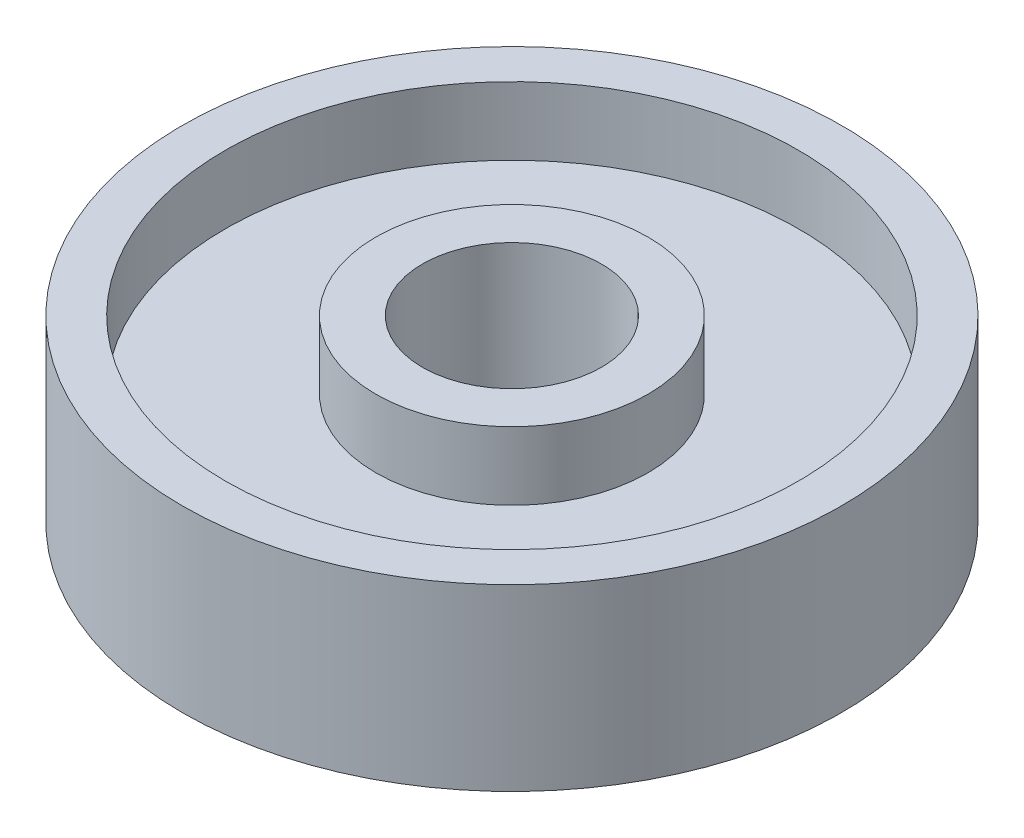
ISO-10303-21;
HEADER;
FILE_DESCRIPTION(('STEP AP214'),'2;1');
FILE_NAME('part.step','',(''),(''),'','','');
FILE_SCHEMA(('AUTOMOTIVE_DESIGN { 1 0 10303 214 1 1 1 1 }'));
ENDSEC;
DATA;
#1=APPLICATION_CONTEXT('core data for automotive mechanical design processes');
#2=APPLICATION_PROTOCOL_DEFINITION('international standard','automotive_design',2000,#1);
#3=PRODUCT_CONTEXT('',#1,'mechanical');
#4=PRODUCT('Part','Part','',(#3));
#5=PRODUCT_RELATED_PRODUCT_CATEGORY('part','',(#4));
#6=PRODUCT_DEFINITION_FORMATION('','',#4);
#7=PRODUCT_DEFINITION_CONTEXT('part definition',#1,'design');
#8=PRODUCT_DEFINITION('design','',#6,#7);
#9=PRODUCT_DEFINITION_SHAPE('','',#8);
#10=(LENGTH_UNIT() NAMED_UNIT(*) SI_UNIT(.MILLI.,.METRE.));
#11=(NAMED_UNIT(*) PLANE_ANGLE_UNIT() SI_UNIT($,.RADIAN.));
#12=(NAMED_UNIT(*) SI_UNIT($,.STERADIAN.) SOLID_ANGLE_UNIT());
#13=UNCERTAINTY_MEASURE_WITH_UNIT(LENGTH_MEASURE(1.E-05),#10,'distance_accuracy_value','');
#14=(GEOMETRIC_REPRESENTATION_CONTEXT(3) GLOBAL_UNCERTAINTY_ASSIGNED_CONTEXT((#13)) GLOBAL_UNIT_ASSIGNED_CONTEXT((#10,
#11,#12)) REPRESENTATION_CONTEXT('',''));
#15=CARTESIAN_POINT('',(0.,0.,0.));
#16=DIRECTION('',(0.,0.,1.));
#17=DIRECTION('',(1.,0.,0.));
#18=AXIS2_PLACEMENT_3D('',#15,#16,#17);
#19=CARTESIAN_POINT('',(0.,3.,0.));
#20=DIRECTION('',(0.,-1.,0.));
#21=DIRECTION('',(0.,0.,-1.));
#22=AXIS2_PLACEMENT_3D('',#19,#20,#21);
#23=CYLINDRICAL_SURFACE('',#22,46.);
#24=CARTESIAN_POINT('',(0.,12.5,0.));
#25=DIRECTION('',(0.,1.,0.));
#26=DIRECTION('',(0.,0.,1.));
#27=AXIS2_PLACEMENT_3D('',#24,#25,#26);
#28=CIRCLE('',#27,46.);
#29=CARTESIAN_POINT('',(0.,12.5,46.));
#30=VERTEX_POINT('',#29);
#31=EDGE_CURVE('E61',#30,#30,#28,.T.);
#32=ORIENTED_EDGE('',*,*,#31,.F.);
#33=EDGE_LOOP('',(#32));
#34=FACE_BOUND('',#33,.T.);
#35=CARTESIAN_POINT('',(0.,-12.5,0.));
#36=DIRECTION('',(0.,1.,0.));
#37=DIRECTION('',(0.,0.,1.));
#38=AXIS2_PLACEMENT_3D('',#35,#36,#37);
#39=CIRCLE('',#38,46.);
#40=CARTESIAN_POINT('',(0.,-12.5,46.));
#41=VERTEX_POINT('',#40);
#42=EDGE_CURVE('E56',#41,#41,#39,.T.);
#43=ORIENTED_EDGE('',*,*,#42,.T.);
#44=EDGE_LOOP('',(#43));
#45=FACE_BOUND('',#44,.T.);
#46=ADVANCED_FACE('F39',(#34,#45),#23,.T.);
#47=CARTESIAN_POINT('',(0.,12.5,0.));
#48=DIRECTION('',(0.,1.,0.));
#49=DIRECTION('',(0.,0.,1.));
#50=AXIS2_PLACEMENT_3D('',#47,#48,#49);
#51=PLANE('',#50);
#52=ORIENTED_EDGE('',*,*,#31,.T.);
#53=EDGE_LOOP('',(#52));
#54=FACE_BOUND('',#53,.T.);
#55=CARTESIAN_POINT('',(0.,12.5,0.));
#56=DIRECTION('',(0.,1.,0.));
#57=DIRECTION('',(0.,0.,1.));
#58=AXIS2_PLACEMENT_3D('',#55,#56,#57);
#59=CIRCLE('',#58,40.);
#60=CARTESIAN_POINT('',(0.,12.5,40.));
#61=VERTEX_POINT('',#60);
#62=EDGE_CURVE('E64',#61,#61,#59,.T.);
#63=ORIENTED_EDGE('',*,*,#62,.F.);
#64=EDGE_LOOP('',(#63));
#65=FACE_BOUND('',#64,.T.);
#66=ADVANCED_FACE('F87',(#54,#65),#51,.T.);
#67=CARTESIAN_POINT('',(0.,12.5,0.));
#68=DIRECTION('',(0.,-1.,0.));
#69=DIRECTION('',(0.,0.,-1.));
#70=AXIS2_PLACEMENT_3D('',#67,#68,#69);
#71=CYLINDRICAL_SURFACE('',#70,40.);
#72=ORIENTED_EDGE('',*,*,#62,.T.);
#73=EDGE_LOOP('',(#72));
#74=FACE_BOUND('',#73,.T.);
#75=CARTESIAN_POINT('',(0.,3.,0.));
#76=DIRECTION('',(0.,1.,0.));
#77=DIRECTION('',(0.,0.,1.));
#78=AXIS2_PLACEMENT_3D('',#75,#76,#77);
#79=CIRCLE('',#78,40.);
#80=CARTESIAN_POINT('',(0.,3.,40.));
#81=VERTEX_POINT('',#80);
#82=EDGE_CURVE('E51',#81,#81,#79,.F.);
#83=ORIENTED_EDGE('',*,*,#82,.T.);
#84=EDGE_LOOP('',(#83));
#85=FACE_BOUND('',#84,.T.);
#86=ADVANCED_FACE('F72',(#74,#85),#71,.F.);
#87=CARTESIAN_POINT('',(0.,3.,0.));
#88=DIRECTION('',(0.,1.,0.));
#89=DIRECTION('',(0.,0.,1.));
#90=AXIS2_PLACEMENT_3D('',#87,#88,#89);
#91=PLANE('',#90);
#92=CARTESIAN_POINT('',(0.,3.,0.));
#93=DIRECTION('',(0.,1.,0.));
#94=DIRECTION('',(0.,0.,1.));
#95=AXIS2_PLACEMENT_3D('',#92,#93,#94);
#96=CIRCLE('',#95,19.);
#97=CARTESIAN_POINT('',(0.,3.,19.));
#98=VERTEX_POINT('',#97);
#99=EDGE_CURVE('E10',#98,#98,#96,.T.);
#100=ORIENTED_EDGE('',*,*,#99,.F.);
#101=EDGE_LOOP('',(#100));
#102=FACE_BOUND('',#101,.T.);
#103=ORIENTED_EDGE('',*,*,#82,.F.);
#104=EDGE_LOOP('',(#103));
#105=FACE_BOUND('',#104,.T.);
#106=ADVANCED_FACE('F71',(#102,#105),#91,.T.);
#107=CARTESIAN_POINT('',(0.,-12.5,0.));
#108=DIRECTION('',(0.,-1.,0.));
#109=DIRECTION('',(0.,0.,1.));
#110=AXIS2_PLACEMENT_3D('',#107,#108,#109);
#111=PLANE('',#110);
#112=CARTESIAN_POINT('',(0.,-12.5,0.));
#113=DIRECTION('',(0.,1.,0.));
#114=DIRECTION('',(0.,0.,1.));
#115=AXIS2_PLACEMENT_3D('',#112,#113,#114);
#116=CIRCLE('',#115,40.);
#117=CARTESIAN_POINT('',(0.,-12.5,40.));
#118=VERTEX_POINT('',#117);
#119=EDGE_CURVE('E57',#118,#118,#116,.T.);
#120=ORIENTED_EDGE('',*,*,#119,.T.);
#121=EDGE_LOOP('',(#120));
#122=FACE_BOUND('',#121,.T.);
#123=ORIENTED_EDGE('',*,*,#42,.F.);
#124=EDGE_LOOP('',(#123));
#125=FACE_BOUND('',#124,.T.);
#126=ADVANCED_FACE('F73',(#122,#125),#111,.T.);
#127=CARTESIAN_POINT('',(0.,-12.5,0.));
#128=DIRECTION('',(0.,1.,0.));
#129=DIRECTION('',(0.,0.,1.));
#130=AXIS2_PLACEMENT_3D('',#127,#128,#129);
#131=CYLINDRICAL_SURFACE('',#130,40.);
#132=ORIENTED_EDGE('',*,*,#119,.F.);
#133=EDGE_LOOP('',(#132));
#134=FACE_BOUND('',#133,.T.);
#135=CARTESIAN_POINT('',(0.,-3.,0.));
#136=DIRECTION('',(0.,1.,0.));
#137=DIRECTION('',(0.,0.,1.));
#138=AXIS2_PLACEMENT_3D('',#135,#136,#137);
#139=CIRCLE('',#138,40.);
#140=CARTESIAN_POINT('',(0.,-3.,40.));
#141=VERTEX_POINT('',#140);
#142=EDGE_CURVE('E46',#141,#141,#139,.T.);
#143=ORIENTED_EDGE('',*,*,#142,.T.);
#144=EDGE_LOOP('',(#143));
#145=FACE_BOUND('',#144,.T.);
#146=ADVANCED_FACE('F81',(#134,#145),#131,.F.);
#147=CARTESIAN_POINT('',(0.,-3.,0.));
#148=DIRECTION('',(0.,1.,0.));
#149=DIRECTION('',(0.,0.,1.));
#150=AXIS2_PLACEMENT_3D('',#147,#148,#149);
#151=PLANE('',#150);
#152=CARTESIAN_POINT('',(0.,-3.,0.));
#153=DIRECTION('',(0.,1.,0.));
#154=DIRECTION('',(0.,0.,1.));
#155=AXIS2_PLACEMENT_3D('',#152,#153,#154);
#156=CIRCLE('',#155,19.);
#157=CARTESIAN_POINT('',(0.,-3.,19.));
#158=VERTEX_POINT('',#157);
#159=EDGE_CURVE('E45',#158,#158,#156,.T.);
#160=ORIENTED_EDGE('',*,*,#159,.T.);
#161=EDGE_LOOP('',(#160));
#162=FACE_BOUND('',#161,.T.);
#163=ORIENTED_EDGE('',*,*,#142,.F.);
#164=EDGE_LOOP('',(#163));
#165=FACE_BOUND('',#164,.T.);
#166=ADVANCED_FACE('F110',(#162,#165),#151,.F.);
#167=CARTESIAN_POINT('',(0.,-12.5,0.));
#168=DIRECTION('',(0.,1.,0.));
#169=DIRECTION('',(0.,0.,1.));
#170=AXIS2_PLACEMENT_3D('',#167,#168,#169);
#171=CYLINDRICAL_SURFACE('',#170,19.);
#172=CARTESIAN_POINT('',(0.,-12.5,0.));
#173=DIRECTION('',(0.,1.,0.));
#174=DIRECTION('',(0.,0.,1.));
#175=AXIS2_PLACEMENT_3D('',#172,#173,#174);
#176=CIRCLE('',#175,19.);
#177=CARTESIAN_POINT('',(0.,-12.5,19.));
#178=VERTEX_POINT('',#177);
#179=EDGE_CURVE('E131',#178,#178,#176,.T.);
#180=ORIENTED_EDGE('',*,*,#179,.T.);
#181=EDGE_LOOP('',(#180));
#182=FACE_BOUND('',#181,.T.);
#183=ORIENTED_EDGE('',*,*,#159,.F.);
#184=EDGE_LOOP('',(#183));
#185=FACE_BOUND('',#184,.T.);
#186=ADVANCED_FACE('F111',(#182,#185),#171,.T.);
#187=CARTESIAN_POINT('',(0.,-12.5,0.));
#188=DIRECTION('',(0.,1.,0.));
#189=DIRECTION('',(0.,0.,1.));
#190=AXIS2_PLACEMENT_3D('',#187,#188,#189);
#191=PLANE('',#190);
#192=CARTESIAN_POINT('',(0.,-12.5,0.));
#193=DIRECTION('',(0.,1.,0.));
#194=DIRECTION('',(0.,0.,1.));
#195=AXIS2_PLACEMENT_3D('',#192,#193,#194);
#196=CIRCLE('',#195,12.5);
#197=CARTESIAN_POINT('',(0.,-12.5,12.5));
#198=VERTEX_POINT('',#197);
#199=EDGE_CURVE('E129',#198,#198,#196,.T.);
#200=ORIENTED_EDGE('',*,*,#199,.T.);
#201=EDGE_LOOP('',(#200));
#202=FACE_BOUND('',#201,.T.);
#203=ORIENTED_EDGE('',*,*,#179,.F.);
#204=EDGE_LOOP('',(#203));
#205=FACE_BOUND('',#204,.T.);
#206=ADVANCED_FACE('F117',(#202,#205),#191,.F.);
#207=CARTESIAN_POINT('',(0.,-12.5,0.));
#208=DIRECTION('',(0.,1.,0.));
#209=DIRECTION('',(0.,0.,1.));
#210=AXIS2_PLACEMENT_3D('',#207,#208,#209);
#211=CYLINDRICAL_SURFACE('',#210,12.5);
#212=ORIENTED_EDGE('',*,*,#199,.F.);
#213=EDGE_LOOP('',(#212));
#214=FACE_BOUND('',#213,.T.);
#215=CARTESIAN_POINT('',(0.,12.5,0.));
#216=DIRECTION('',(0.,1.,0.));
#217=DIRECTION('',(0.,0.,1.));
#218=AXIS2_PLACEMENT_3D('',#215,#216,#217);
#219=CIRCLE('',#218,12.5);
#220=CARTESIAN_POINT('',(0.,12.5,12.5));
#221=VERTEX_POINT('',#220);
#222=EDGE_CURVE('E134',#221,#221,#219,.T.);
#223=ORIENTED_EDGE('',*,*,#222,.T.);
#224=EDGE_LOOP('',(#223));
#225=FACE_BOUND('',#224,.T.);
#226=ADVANCED_FACE('F114',(#214,#225),#211,.F.);
#227=ORIENTED_EDGE('',*,*,#99,.T.);
#228=EDGE_LOOP('',(#227));
#229=FACE_BOUND('',#228,.T.);
#230=CARTESIAN_POINT('',(0.,12.5,0.));
#231=DIRECTION('',(0.,1.,0.));
#232=DIRECTION('',(0.,0.,1.));
#233=AXIS2_PLACEMENT_3D('',#230,#231,#232);
#234=CIRCLE('',#233,19.);
#235=CARTESIAN_POINT('',(0.,12.5,19.));
#236=VERTEX_POINT('',#235);
#237=EDGE_CURVE('E53',#236,#236,#234,.T.);
#238=ORIENTED_EDGE('',*,*,#237,.F.);
#239=EDGE_LOOP('',(#238));
#240=FACE_BOUND('',#239,.T.);
#241=ADVANCED_FACE('F108',(#229,#240),#171,.T.);
#242=CARTESIAN_POINT('',(0.,12.5,0.));
#243=DIRECTION('',(0.,1.,0.));
#244=DIRECTION('',(0.,0.,1.));
#245=AXIS2_PLACEMENT_3D('',#242,#243,#244);
#246=PLANE('',#245);
#247=ORIENTED_EDGE('',*,*,#222,.F.);
#248=EDGE_LOOP('',(#247));
#249=FACE_BOUND('',#248,.T.);
#250=ORIENTED_EDGE('',*,*,#237,.T.);
#251=EDGE_LOOP('',(#250));
#252=FACE_BOUND('',#251,.T.);
#253=ADVANCED_FACE('F115',(#249,#252),#246,.T.);
#254=CLOSED_SHELL('',(#46,#66,#86,#106,#126,#146,#166,#186,#206,#226,#241,#253));
#255=MANIFOLD_SOLID_BREP('B2',#254);
#256=ADVANCED_BREP_SHAPE_REPRESENTATION('',(#18,#255),#14);
#257=SHAPE_DEFINITION_REPRESENTATION(#9,#256);
ENDSEC;
END-ISO-10303-21;
